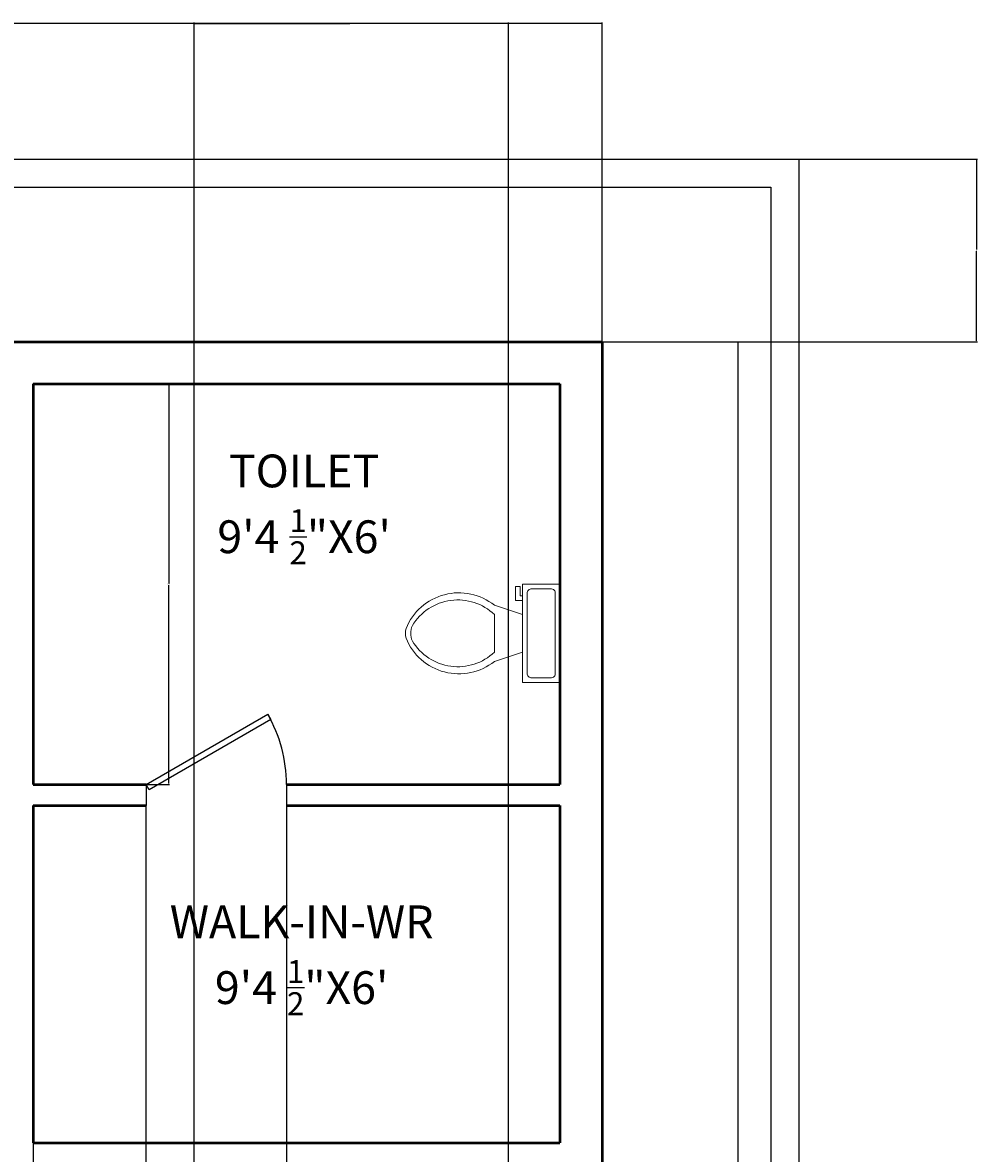
# Model space of a CAD drawing. Units: inches. Extents: x -28 to 483, y -584 to 51.
# Tile 6 of 6: x 279 to 483, y -191 to 51. Entities that reach past the tile are written whole.
import ezdxf

# ---------------------------------------------------------------- set-up
doc = ezdxf.new("R2010")
doc.units = ezdxf.units.IN
doc.header["$MEASUREMENT"] = 0
for name, color, linetype, lineweight in [('A-ANNO-DIMS', 2, 'Continuous', 18), ('A-AREA-IDEN', 7, 'Continuous', 25), ('A-DOOR', 4, 'Continuous', 25), ('A-FLOR-FIXT', 9, 'Continuous', 18), ('A-WALL', 7, 'Continuous', 50), ('C-PROP', 7, 'Continuous', 25)]:
    doc.layers.add(name, color=color, linetype=linetype, lineweight=lineweight)
doc.styles.get("Standard").update_dxf_attribs({"font": 'arial.ttf'})
doc.dimstyles.get("Standard").update_dxf_attribs({"dimtxt": 0.18, "dimasz": 0.18, "dimexe": 0.18, "dimexo": 0.0625, "dimgap": 0.09, "dimtad": 0, "dimtih": 1, "dimtoh": 1, "dimdec": 4, "dimzin": 0, "dimdsep": 46, "dimtxsty": 'Standard', "dimcen": 0.09, "dimadec": 0, "dimazin": 0, "dimtfac": 1, "dimtdec": 4, "dimtofl": 0, "dimtmove": 0, "dimatfit": 3, "dimfxl": 1, "dimtolj": 1, "dimtzin": 0, "dimarcsym": 0})

# ---------------------------------------------------------------- blocks, each defined once
blk = doc.blocks.new('*U2')
for p, q in [((0, 0), (0, -6)), ((40, 0), (40, -6))]:
    blk.add_line(p, q)
blk.add_lwpolyline([(0, 0), (34.64, 20), (35.52, 18.48), (0.87, -1.52)], close=True)
blk.add_arc((0, 0), 40, 0, 30)
blk = doc.blocks.new('*U5')
for p, q in [((9.5, -6), (9.5, -2)), ((-10, -8.5), (-8, -8.5)), ((-10, -9.5), (-10, -8.5)), ((-7, -9.5), (-10, -9.5)), ((-8, -8.5), (-8, -8)), ((-7, -8), (-7, -9.5)), ((-4, -8), (-6, -14)), ((4, -8), (6, -14)), ((4, -14), (-4, -14))]:
    blk.add_line(p, q)
blk.add_lwpolyline([(10.5, -8), (10.5, 0), (-10.5, 0), (-10.5, -8)], close=True)
for points in [[(-9.5, -2), (-9.5, -6)], [(8.5, -1), (-8.5, -1)], [(-8.5, -7), (8.5, -7)]]:
    blk.add_lwpolyline(points)
for centre, radius, start, end in [((-8.62, -1.88), 0.884, 81.8699, 188.1301), ((8.62, -1.88), 0.884, 351.8699, 98.1301), ((-8.62, -6.12), 0.884, 171.8699, 278.1301), ((8.62, -6.12), 0.884, 261.8699, 8.1301), ((3.52, -21.58), 12.17, 141.4691, 247.9714), ((4.2, -21.82), 11.33, 136.3677, 238.9468), ((-3.52, -21.58), 12.17, 292.0284, 38.5307), ((-4.2, -21.82), 11.33, 301.053, 43.6321), ((0, -27.88), 4, 245.7318, 294.2682), ((0, -29), 4, 254.8605, 285.1395)]:
    blk.add_arc(centre, radius, start, end)
blk = doc.blocks.new('*D21')
at = {"layer": 'A-ANNO-DIMS', "color": 0, "lineweight": -2, "transparency": 16777216}
for p, q in [((51.84, -17.53), (51.84, 50.54)), ((52.02, 50.36), (227.07, 50.36)), ((402.66, 50.36), (227.61, 50.36)), ((402.84, -17.53), (402.84, 50.54))]:
    blk.add_line(p, q, dxfattribs=at)
at = {"layer": 'A-ANNO-DIMS', "color": 0, "transparency": 16777216}
for points in [[(52.02, 50.39), (52.02, 50.33), (51.84, 50.36)], [(402.66, 50.39), (402.66, 50.33), (402.84, 50.36)]]:
    blk.add_solid(points, dxfattribs=at)
at = {"layer": 'Defpoints', "color": 0, "transparency": 16777216}
for p in [(402.84, 50.36), (51.84, -17.59), (402.84, -17.59)]:
    blk.add_point(p, dxfattribs=at)
at = {"layer": 'A-ANNO-DIMS', "color": 0, "transparency": 16777216, "insert": (227.34, 50.36), "char_height": 0.18, "attachment_point": 5}
blk.add_mtext('\\A1;351', dxfattribs=at)
blk = doc.blocks.new('*D22')
at = {"layer": 'A-ANNO-DIMS', "color": 0, "lineweight": -2, "transparency": 16777216}
for p, q in [((402.905662, -17.587684), (431.973162, -17.587684)), ((431.793162, -17.767684), (431.793162, -255.907684)), ((431.793162, -494.407684), (431.793162, -256.267684)), ((402.905662, -494.587684), (431.973162, -494.587684))]:
    blk.add_line(p, q, dxfattribs=at)
at = {"layer": 'A-ANNO-DIMS', "color": 0, "transparency": 16777216}
for points in [[(431.763162, -17.767684), (431.823162, -17.767684), (431.793162, -17.587684)], [(431.763162, -494.407684), (431.823162, -494.407684), (431.793162, -494.587684)]]:
    blk.add_solid(points, dxfattribs=at)
at = {"layer": 'Defpoints', "color": 0, "transparency": 16777216}
for p in [(402.843162, -17.587684), (402.843162, -494.587684), (431.793162, -494.587684)]:
    blk.add_point(p, dxfattribs=at)
at = {"layer": 'A-ANNO-DIMS', "color": 0, "transparency": 16777216, "insert": (431.793162, -256.087684), "char_height": 0.18, "attachment_point": 5}
blk.add_mtext('\\A1;477', dxfattribs=at)
blk = doc.blocks.new('*D24')
at = {"layer": 'A-ANNO-DIMS', "color": 0, "lineweight": -2, "transparency": 16777216}
for p, q in [((444.91, 21.41), (482.97, 21.41)), ((482.79, 21.23), (482.79, 2.09)), ((482.79, -17.41), (482.79, 1.73)), ((402.91, -17.59), (482.97, -17.59))]:
    blk.add_line(p, q, dxfattribs=at)
at = {"layer": 'A-ANNO-DIMS', "color": 0, "transparency": 16777216}
for points in [[(482.76, 21.23), (482.82, 21.23), (482.79, 21.41)], [(482.76, -17.41), (482.82, -17.41), (482.79, -17.59)]]:
    blk.add_solid(points, dxfattribs=at)
at = {"layer": 'Defpoints', "color": 0, "transparency": 16777216}
for p in [(444.84, 21.41), (402.84, -17.59), (482.79, -17.59)]:
    blk.add_point(p, dxfattribs=at)
at = {"layer": 'A-ANNO-DIMS', "color": 0, "transparency": 16777216, "insert": (482.79, 1.91), "char_height": 0.18, "attachment_point": 5}
blk.add_mtext('\\A1;39', dxfattribs=at)
blk = doc.blocks.new('*D25')
at = {"layer": 'A-ANNO-DIMS', "color": 0, "lineweight": -2, "transparency": 16777216}
for p, q in [((281.41, -26.59), (310.47, -26.59)), ((310.29, -26.77), (310.29, -69.16)), ((310.29, -111.91), (310.29, -69.52)), ((281.41, -112.09), (310.47, -112.09))]:
    blk.add_line(p, q, dxfattribs=at)
at = {"layer": 'A-ANNO-DIMS', "color": 0, "transparency": 16777216}
for points in [[(310.26, -26.77), (310.32, -26.77), (310.29, -26.59)], [(310.26, -111.91), (310.32, -111.91), (310.29, -112.09)]]:
    blk.add_solid(points, dxfattribs=at)
at = {"layer": 'Defpoints', "color": 0, "transparency": 16777216}
for p in [(281.34, -26.59), (281.34, -112.09), (310.29, -112.09)]:
    blk.add_point(p, dxfattribs=at)
at = {"layer": 'A-ANNO-DIMS', "color": 0, "transparency": 16777216, "insert": (310.29, -69.34), "char_height": 0.18, "attachment_point": 5}
blk.add_mtext('\\A1;85.5', dxfattribs=at)
blk = doc.blocks.new('*D30')
at = {"layer": 'A-ANNO-DIMS', "color": 0, "lineweight": -2, "transparency": 16777216}
for p, q in [((305.44, -116.65), (305.44, -583.72)), ((335.44, -116.65), (335.44, -583.72)), ((305.62, -583.54), (320.22, -583.54)), ((335.26, -583.54), (320.66, -583.54))]:
    blk.add_line(p, q, dxfattribs=at)
at = {"layer": 'A-ANNO-DIMS', "color": 0, "transparency": 16777216}
for points in [[(305.62, -583.51), (305.62, -583.57), (305.44, -583.54)], [(335.26, -583.51), (335.26, -583.57), (335.44, -583.54)]]:
    blk.add_solid(points, dxfattribs=at)
at = {"layer": 'Defpoints', "color": 0, "transparency": 16777216}
for p in [(305.44, -116.59), (335.44, -116.59), (335.44, -583.54)]:
    blk.add_point(p, dxfattribs=at)
at = {"layer": 'A-ANNO-DIMS', "color": 0, "transparency": 16777216, "insert": (320.44, -583.54), "char_height": 0.18, "attachment_point": 5}
blk.add_mtext('\\A1;30', dxfattribs=at)
blk = doc.blocks.new('*D31')
at = {"layer": 'A-ANNO-DIMS', "color": 0, "lineweight": -2, "transparency": 16777216}
for p, q in [((281.34, -116.65), (281.34, -583.72)), ((305.44, -116.65), (305.44, -583.72)), ((281.52, -583.54), (293.08, -583.54)), ((305.26, -583.54), (293.7, -583.54))]:
    blk.add_line(p, q, dxfattribs=at)
at = {"layer": 'A-ANNO-DIMS', "color": 0, "transparency": 16777216}
for points in [[(281.52, -583.51), (281.52, -583.57), (281.34, -583.54)], [(305.26, -583.51), (305.26, -583.57), (305.44, -583.54)]]:
    blk.add_solid(points, dxfattribs=at)
at = {"layer": 'Defpoints', "color": 0, "transparency": 16777216}
for p in [(281.34, -116.59), (305.44, -116.59), (305.44, -583.54)]:
    blk.add_point(p, dxfattribs=at)
at = {"layer": 'A-ANNO-DIMS', "color": 0, "transparency": 16777216, "insert": (293.39, -583.54), "char_height": 0.18, "attachment_point": 5}
blk.add_mtext('\\A1;24.1', dxfattribs=at)
blk = doc.blocks.new('*D41')
at = {"layer": 'A-ANNO-DIMS', "color": 0, "lineweight": -2, "transparency": 16777216}
for p, q in [((315.72, -337.03), (315.72, 50.54)), ((315.9, 50.36), (348.97, 50.36)), ((382.64, 50.36), (349.58, 50.36)), ((382.82, -337.03), (382.82, 50.54))]:
    blk.add_line(p, q, dxfattribs=at)
at = {"layer": 'A-ANNO-DIMS', "color": 0, "transparency": 16777216}
for points in [[(315.9, 50.39), (315.9, 50.33), (315.72, 50.36)], [(382.64, 50.39), (382.64, 50.33), (382.82, 50.36)]]:
    blk.add_solid(points, dxfattribs=at)
at = {"layer": 'Defpoints', "color": 0, "transparency": 16777216}
for p in [(382.82, 50.36), (315.72, -337.09), (382.82, -337.09)]:
    blk.add_point(p, dxfattribs=at)
at = {"layer": 'A-ANNO-DIMS', "color": 0, "transparency": 16777216, "insert": (349.27, 50.36), "char_height": 0.18, "attachment_point": 5}
blk.add_mtext('\\A1;67.1', dxfattribs=at)

msp = doc.modelspace()

# ---------------------------------------------------------------- linework, layer by layer
at = {"layer": 'A-WALL'}
for p, q in [((51.8432, -17.5877), (402.8432, -17.5877)), ((402.8432, -17.5877), (402.8432, -494.5877)), ((281.3432, -26.5877), (281.3432, -112.0877)), ((281.3432, -26.5877), (393.8432, -26.5877)), ((393.8432, -26.5877), (393.8432, -112.0877)), ((281.3432, -112.0877), (305.4421, -112.0877)), ((335.4421, -112.0877), (393.8432, -112.0877)), ((281.3432, -116.5877), (305.4421, -116.5877)), ((281.3432, -116.5877), (281.3432, -188.5877)), ((335.4421, -116.5877), (393.8432, -116.5877)), ((393.8432, -116.5877), (393.8432, -188.5877)), ((281.3432, -188.5877), (393.8432, -188.5877))]:
    msp.add_line(p, q, dxfattribs=at)
at = {"layer": 'C-PROP'}
for p, q in [((12.8432, 21.4123), (444.8432, 21.4123)), ((444.8432, 21.4123), (444.8432, -554.5877)), ((18.8432, 15.4123), (438.8432, 15.4123)), ((438.8432, 15.4123), (438.8432, -548.5877))]:
    msp.add_line(p, q, dxfattribs=at)

# ---------------------------------------------------------------- block references
at = {"layer": 'A-DOOR', "xscale": 0.75, "yscale": 0.75, "zscale": 0.75}
msp.add_blockref('*U2', (305.4421, -112.0877), dxfattribs=at)
at = {"layer": 'A-FLOR-FIXT', "rotation": 270}
msp.add_blockref('*U5', (393.8432, -79.822), dxfattribs=at)

# ---------------------------------------------------------------- texts
at = {"layer": 'A-AREA-IDEN', "char_height": 7, "attachment_point": 1}
for s, insert in [('\\A1;\\pxqc;TOILET\\P9\'4 {\\H0.7x;\\S1/2;}"X6\'', (288.4927, -41.6592)), ('\\A1;\\pxqc;WALK-IN-WR\\P9\'4 {\\H0.7x;\\S1/2;}"X6\'', (287.967, -137.9066))]:
    msp.add_mtext_dynamic_manual_height_columns(s, width=101.426885, gutter_width=1, heights=[0], dxfattribs=dict(at, insert=insert))

# ---------------------------------------------------------------- dimensions: what is measured, and where the dimension line sits
at = {"layer": 'A-ANNO-DIMS'}
for base, p1, p2, override, picture, middle in [((402.8432, 50.3623), (51.8432, -17.5877), (402.8432, -17.5877), {"dimdec": 0, "dimlfac": 1, "dimrnd": 0, "dimzin": 0, "dimdsep": 46, "dimlunit": 2}, '*D21', (227.3432, 50.3623)), ((382.8208, 50.3623), (315.7242, -337.0877), (382.8208, -337.0877), {"dimdec": 1, "dimlfac": 1, "dimrnd": 0, "dimzin": 0, "dimdsep": 46, "dimlunit": 2}, '*D41', (349.2725, 50.3623)), ((305.4421, -583.5377), (281.3432, -116.5877), (305.4421, -116.5877), {"dimdec": 1, "dimlfac": 1, "dimrnd": 0, "dimzin": 0, "dimdsep": 46, "dimlunit": 2}, '*D31', (293.3926, -583.5377)), ((335.4421, -583.5377), (305.4421, -116.5877), (335.4421, -116.5877), {"dimdec": 0, "dimlfac": 1, "dimrnd": 0, "dimzin": 0, "dimdsep": 46, "dimlunit": 2}, '*D30', (320.4421, -583.5377))]:
    dim = msp.add_linear_dim(base=base, p1=p1, p2=p2, dimstyle='Standard', override=override, dxfattribs=at)
    dim.commit()
    dim.dimension.update_dxf_attribs({"geometry": picture, "text_midpoint": middle})
for base, p1, p2, angle, override, picture, middle in [((482.7932, -17.5877), (444.8432, 21.4123), (402.8432, -17.5877), 90, {"dimdec": 0, "dimlfac": 1, "dimrnd": 0, "dimzin": 0, "dimdsep": 46, "dimlunit": 2}, '*D24', (482.7932, 1.9123)), ((431.7932, -494.5877), (402.8432, -17.5877), (402.8432, -494.5877), 270, {"dimdec": 0, "dimlfac": 1, "dimrnd": 0, "dimzin": 0, "dimdsep": 46, "dimlunit": 2}, '*D22', (431.7932, -256.0877)), ((310.2932, -112.0877), (281.3432, -26.5877), (281.3432, -112.0877), 270, {"dimdec": 1, "dimlfac": 1, "dimrnd": 0, "dimzin": 0, "dimdsep": 46, "dimlunit": 2}, '*D25', (310.2932, -69.3377))]:
    dim = msp.add_linear_dim(base=base, p1=p1, p2=p2, angle=angle, dimstyle='Standard', override=override, dxfattribs=at)
    dim.commit()
    dim.dimension.update_dxf_attribs({"geometry": picture, "text_midpoint": middle})

doc.saveas('drawing.dxf')
